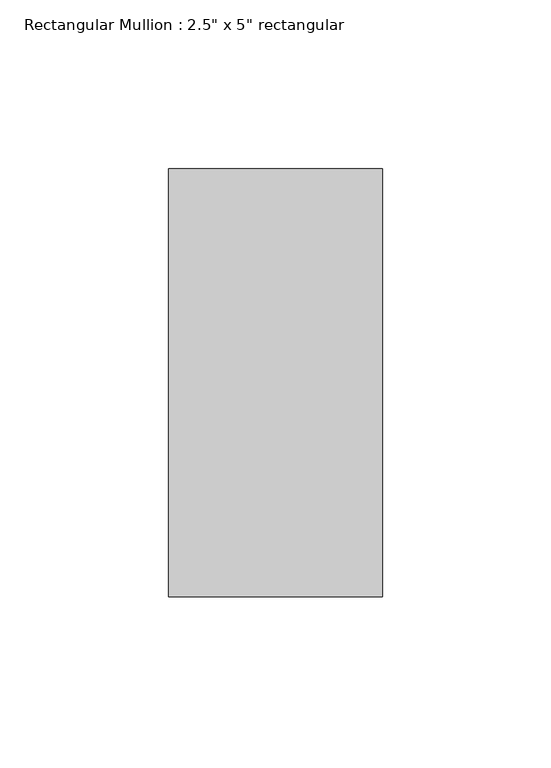
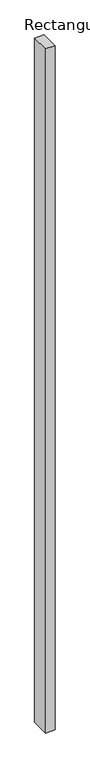
"""IFC4 building model written with IfcOpenShell, lengths in millimetres: member geometry."""

from ifc_helpers import new_model, si_unit, frame, origin, place, context, project, spatial, polyline, outline, extrude, source, transform, mapped, element, save


def member_5d32774f(model_context):
    return source(origin(), model_context, "Body", "SweptSolid", [
        extrude(outline(polyline([(0.0, 63.5), (0.0, -63.5), (-63.5, -63.5), (-63.5, 63.5), (0.0, 63.5)])), frame((0.0, 0.0, -4851.4), z_axis=(0.0, 0.0, 1.0), x_axis=(1.0, 0.0, 0.0)), (0.0, 0.0, 1.0), 4851.4),
    ])


if __name__ == "__main__":
    model = new_model("IFC4")
    model_context = context("Model", 3, world=origin())
    ifc_project = project(units=[si_unit("LENGTHUNIT", "METRE", prefix="MILLI")], contexts=[model_context])
    site = spatial("IfcSite", under=ifc_project)
    building = spatial("IfcBuilding", under=site)
    placement = place(None, origin())
    member_shape = member_5d32774f(model_context)
    element("IfcMember", 1, ObjectType="Rectangular Mullion : 2.5\" x 5\" rectangular", at=placement, inside=building, context=model_context, shape_type="MappedRepresentation", body=[
        mapped(member_shape, transform((0.0, 0.0, 0.0), x_axis=(1.0, 0.0, 0.0), y_axis=(0.0, 1.0, 0.0), z_axis=(0.0, 0.0, 1.0))),
    ])
    save(model, "model.ifc")

# Revit data of these elements
# Type "Rectangular Mullion : 2.5\" x 5\" rectangular"
#   built-in parameter 1007304 = 0.416667 (stored number, unit not read)
#   built-in parameter 1007301 = 0.104167 (stored number, unit not read)
#   built-in parameter 1007300 = 0.104167 (stored number, unit not read)
# Element 1 (IfcMember, "Rectangular Mullion : 2.5\" x 5\" rectangular")
#   Materials on its faces: "Aluminum"
# Materials
#   "Aluminum": class "Metal", colour RGB 247 247 247, transparency 0, Description = "Aluminum 6061", Cost = 0
